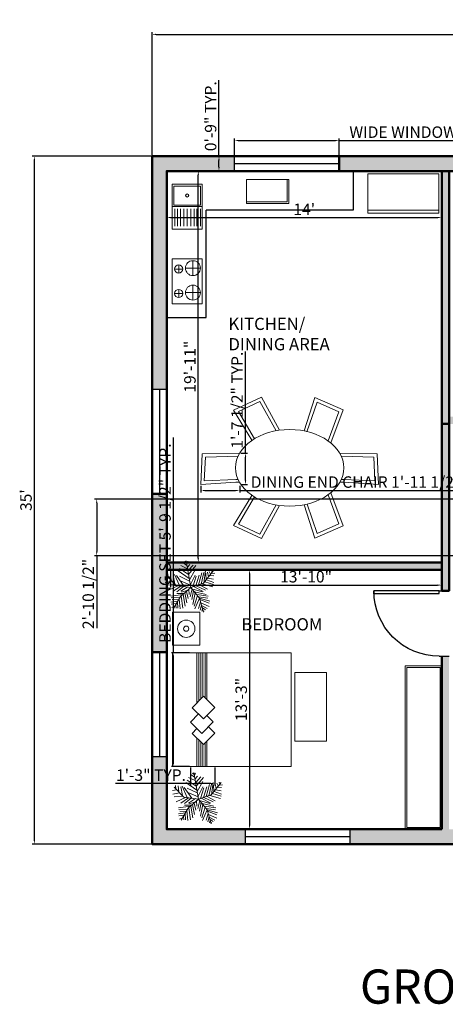
# Model space of a CAD drawing. Units: inches. Extents: x 1647 to 2354, y 1705 to 2321.
# Tile 1 of 4: x 1647 to 1907, y 1705 to 2307. Entities that reach past the tile are written whole.
import ezdxf

# ---------------------------------------------------------------- set-up
doc = ezdxf.new("R2010")
doc.units = ezdxf.units.IN
for name, color, linetype, lineweight in [('A-ANNO-DIMS', 130, 'Continuous', 18), ('A-ANNO-TEXT', 7, 'Continuous', 35), ('A-AREA-IDEN', 7, 'Continuous', 25), ('A-EQPM', 52, 'Continuous', 18), ('A-FLOR-CASE', 52, 'Continuous', 25), ('A-FLOR-FIXT', 52, 'Continuous', 18), ('A-WALL-PATT', 84, 'Continuous', 13), ('door', 142, 'Continuous', 25), ('fur', 52, 'Continuous', 18), ('tree', 92, 'Continuous', 13), ('wall', 84, 'Continuous', 50), ('window', 242, 'Continuous', 25)]:
    doc.layers.add(name, color=color, linetype=linetype, lineweight=lineweight)
doc.styles.get("Standard").update_dxf_attribs({"font": 'arial.ttf'})
doc.dimstyles.new('ISO-25', dxfattribs={"dimtxt": 7, "dimasz": 2.5, "dimexe": 1.25, "dimexo": 0.625, "dimtad": 1, "dimdec": 0, "dimlunit": 4, "dimtxsty": 'Standard', "dimcen": 2.5, "dimadec": 0, "dimazin": 0, "dimtfac": 1, "dimtdec": 0, "dimtmove": 0, "dimatfit": 3, "dimfxl": 1, "dimarcsym": 0})

# ---------------------------------------------------------------- blocks, each defined once
blk = doc.blocks.new('*U2')
for p, q in [((0, 0), (0, -6)), ((40, 0), (40, -6))]:
    blk.add_line(p, q)
blk.add_lwpolyline([(0, 0), (0, 40), (1.75, 40), (1.75, 0)], close=True)
blk.add_arc((0, 0), 40, 0, 90)
blk = doc.blocks.new('*U6')
for p, q in [((-7.288, 39.707), (-21.778, 46.673)), ((-8.737, 47.138), (-17.069, 52.711)), ((-10.186, 53.64), (-13.084, 55.962)), ((0, 0), (-10.5, 57)), ((-9.099, 51.782), (-6.563, 55.962)), ((-7.65, 43.423), (-2.578, 49.46)), ((-5.839, 35.992), (4.667, 48.067)), ((-5.114, 27.632), (10.463, 46.673)), ((-31.5, 4.5), (-52.5, 25.5)), ((-48.585, 21.131), (-49.309, 29.026)), ((-43.513, 28.561), (-42.427, 15.558)), ((-38.442, 26.239), (-34.819, 7.663)), ((-35.544, 28.097), (-24.314, 3.947)), ((-14.533, 2.09), (-30.834, 25.31)), ((-3.665, 19.273), (-27.574, 35.527)), ((-5.114, 28.097), (-24.676, 40.636)), ((-24.314, 23.917), (-2.941, 13.7)), ((-2.941, 16.486), (8.652, 37.85)), ((-1.129, 6.734), (9.014, 26.704)), ((3.942, 1.625), (11.187, 24.381)), ((10.101, 3.483), (17.708, 26.239)), ((16.259, 5.805), (23.142, 31.348)), ((22.055, 7.198), (27.489, 32.277)), ((27, 9), (48, 36)), ((27.127, 9.056), (31.112, 35.992)), ((31.836, 30.883), (32.561, 16.486)), ((35.096, 32.741), (37.27, 22.524)), ((38.719, 34.134), (41.979, 28.561)), ((40.53, 25.775), (48.862, 24.846)), ((43.791, 29.954), (51.036, 30.883)), ((44.153, 36.456), (45.239, 32.741)), ((-47.498, 19.737), (-55.83, 18.344)), ((-40.615, 13.7), (-55.105, 10.913)), ((-33.37, 6.269), (-52.207, 5.34)), ((-28.299, 3.483), (-47.86, -5.805)), ((-21.416, 3.018), (-38.079, -8.128)), ((0, 0), (-31.5, 4.5)), ((-15.982, 2.09), (-30.11, -9.521)), ((0, 0), (-22.5, -19.5)), ((-6.563, 1.161), (-21.416, -8.128)), ((-20.691, 13.7), (-1.129, 4.876)), ((0, 0), (27, 9)), ((0, 0), (18, -22.5)), ((6.478, 1.625), (26.04, -8.592)), ((11.187, 3.483), (30.749, -5.805)), ((18.07, 5.805), (35.096, -3.483)), ((24.229, 7.663), (46.688, 1.625)), ((29.662, 12.307), (48.137, 6.269)), ((33.285, 16.486), (48.862, 10.913)), ((36.183, 19.737), (48.137, 17.88)), ((-17.431, -15.094), (-42.789, -18.809)), ((-22.5, -19.5), (-37.5, -45)), ((-15.257, -12.772), (-30.11, -12.772)), ((-20.691, -18.345), (-17.793, -44.352)), ((-6.563, -5.805), (-19.967, -9.985)), ((-17.069, -15.094), (-12.721, -40.172)), ((-13.446, -11.378), (-8.737, -32.741)), ((-9.461, -8.592), (-6.201, -23.453)), ((-4.752, -3.483), (-3.665, -14.629)), ((2.493, -3.019), (-1.491, -20.202)), ((1.769, -2.555), (24.229, -9.521)), ((5.029, -6.27), (2.131, -25.775)), ((9.014, -11.378), (3.58, -35.992)), ((14.085, -16.951), (6.478, -40.172)), ((7.565, -9.056), (32.198, -14.629)), ((12.274, -15.094), (36.907, -18.809)), ((16.259, -19.738), (36.183, -22.989)), ((-28.299, -29.026), (-42.789, -31.348)), ((-24.314, -21.596), (-42.427, -22.06)), ((-30.834, -34.135), (-42.427, -35.528)), ((-34.457, -39.708), (-40.978, -42.494)), ((-26.849, -26.24), (-40.253, -25.775)), ((-32.646, -36.921), (-31.921, -44.352)), ((-29.023, -30.884), (-27.936, -43.887)), ((-25.038, -23.918), (-22.865, -45.281)), ((18.07, -22.524), (8.289, -45.745)), ((20.244, -30.419), (15.897, -44.816)), ((18, -22.5), (27, -52.5)), ((18.433, -22.524), (40.53, -29.026)), ((19.157, -25.311), (38.719, -33.206)), ((22.78, -37.85), (19.519, -48.532)), ((21.331, -32.741), (39.081, -40.636)), ((22.78, -38.314), (34.372, -44.816)), ((24.591, -45.745), (23.142, -50.854)), ((24.591, -43.423), (30.749, -47.603)), ((26.764, -49.925), (28.213, -50.854))]:
    blk.add_line(p, q)
blk = doc.blocks.new('*D7')
at = {"layer": 'A-ANNO-DIMS', "color": 0, "lineweight": -2, "transparency": 16777216}
for p, q in [((1737.13, 2213.61), (1737.13, 2184.55)), ((1905.13, 2213.61), (1905.13, 2184.55)), ((1739.63, 2185.8), (1902.63, 2185.8))]:
    blk.add_line(p, q, dxfattribs=at)
at = {"layer": 'A-ANNO-DIMS', "color": 0, "transparency": 16777216}
for points in [[(1739.63, 2186.21), (1739.63, 2185.38), (1737.13, 2185.8)], [(1902.63, 2186.21), (1902.63, 2185.38), (1905.13, 2185.8)]]:
    blk.add_solid(points, dxfattribs=at)
at = {"layer": 'Defpoints', "color": 0, "transparency": 16777216}
for p in [(1737.13, 2214.23), (1905.13, 2214.23), (1905.13, 2185.8)]:
    blk.add_point(p, dxfattribs=at)
at = {"layer": 'A-ANNO-DIMS', "color": 0, "transparency": 16777216, "insert": (1821.13, 2189.94), "char_height": 7, "attachment_point": 5}
blk.add_mtext("14'", dxfattribs=at)
blk = doc.blocks.new('*D8')
at = {"layer": 'A-ANNO-DIMS', "color": 0, "lineweight": -2, "transparency": 16777216}
for p, q in [((1737.76, 2214.23), (1757.65, 2214.23)), ((1756.4, 1977.73), (1756.4, 2211.73)), ((1737.76, 1975.23), (1757.65, 1975.23))]:
    blk.add_line(p, q, dxfattribs=at)
at = {"layer": 'A-ANNO-DIMS', "color": 0, "transparency": 16777216}
for points in [[(1755.98, 2211.73), (1756.81, 2211.73), (1756.4, 2214.23)], [(1755.98, 1977.73), (1756.81, 1977.73), (1756.4, 1975.23)]]:
    blk.add_solid(points, dxfattribs=at)
at = {"layer": 'Defpoints', "color": 0, "transparency": 16777216}
for p in [(1737.13, 2214.23), (1756.4, 2214.23), (1737.13, 1975.23)]:
    blk.add_point(p, dxfattribs=at)
at = {"layer": 'A-ANNO-DIMS', "color": 0, "transparency": 16777216, "insert": (1752.2, 2094.73), "char_height": 7, "attachment_point": 5, "rotation": 90}
blk.add_mtext('19\'-11"', dxfattribs=at)
blk = doc.blocks.new('*D13')
at = {"layer": 'A-ANNO-DIMS', "color": 0, "lineweight": -2, "transparency": 16777216}
for p, q in [((1739.39, 1970.11), (1739.39, 1960.1)), ((1905.13, 1970.11), (1905.13, 1960.1)), ((1741.89, 1961.35), (1902.63, 1961.35))]:
    blk.add_line(p, q, dxfattribs=at)
at = {"layer": 'A-ANNO-DIMS', "color": 0, "transparency": 16777216}
for points in [[(1741.89, 1961.76), (1741.89, 1960.93), (1739.39, 1961.35)], [(1902.63, 1961.76), (1902.63, 1960.93), (1905.13, 1961.35)]]:
    blk.add_solid(points, dxfattribs=at)
at = {"layer": 'Defpoints', "color": 0, "transparency": 16777216}
for p in [(1739.39, 1970.73), (1905.13, 1970.73), (1905.13, 1961.35)]:
    blk.add_point(p, dxfattribs=at)
at = {"layer": 'A-ANNO-DIMS', "color": 0, "transparency": 16777216, "insert": (1822.26, 1965.55), "char_height": 7, "attachment_point": 5}
blk.add_mtext('13\'-10"', dxfattribs=at)
blk = doc.blocks.new('*D14')
at = {"layer": 'A-ANNO-DIMS', "color": 0, "lineweight": -2, "transparency": 16777216}
for p, q in [((1737.76, 1970.73), (1788.98, 1970.73)), ((1787.73, 1968.23), (1787.73, 1814.73)), ((1737.76, 1812.23), (1788.98, 1812.23))]:
    blk.add_line(p, q, dxfattribs=at)
at = {"layer": 'A-ANNO-DIMS', "color": 0, "transparency": 16777216}
for points in [[(1787.32, 1968.23), (1788.15, 1968.23), (1787.73, 1970.73)], [(1787.32, 1814.73), (1788.15, 1814.73), (1787.73, 1812.23)]]:
    blk.add_solid(points, dxfattribs=at)
at = {"layer": 'Defpoints', "color": 0, "transparency": 16777216}
for p in [(1737.13, 1970.73), (1737.13, 1812.23), (1787.73, 1812.23)]:
    blk.add_point(p, dxfattribs=at)
at = {"layer": 'A-ANNO-DIMS', "color": 0, "transparency": 16777216, "insert": (1783.53, 1891.48), "char_height": 7, "attachment_point": 5, "rotation": 90}
blk.add_mtext('13\'-3"', dxfattribs=at)
blk = doc.blocks.new('*D24')
at = {"layer": 'A-ANNO-DIMS', "color": 0, "lineweight": -2, "transparency": 16777216}
for p, q in [((1728.13, 2223.86), (1728.13, 2298.93)), ((1730.63, 2297.68), (2265.63, 2297.68)), ((2268.13, 2223.86), (2268.13, 2298.93))]:
    blk.add_line(p, q, dxfattribs=at)
at = {"layer": 'A-ANNO-DIMS', "color": 0, "transparency": 16777216}
for points in [[(1730.63, 2298.09), (1730.63, 2297.26), (1728.13, 2297.68)], [(2265.63, 2298.09), (2265.63, 2297.26), (2268.13, 2297.68)]]:
    blk.add_solid(points, dxfattribs=at)
at = {"layer": 'Defpoints', "color": 0, "transparency": 16777216}
for p in [(2268.13, 2297.68), (1728.13, 2223.23), (2268.13, 2223.23)]:
    blk.add_point(p, dxfattribs=at)
at = {"layer": 'A-ANNO-DIMS', "color": 0, "transparency": 16777216, "insert": (1998.13, 2301.86), "char_height": 7, "attachment_point": 5}
blk.add_mtext("45'", dxfattribs=at)
blk = doc.blocks.new('*D25')
at = {"layer": 'A-ANNO-DIMS', "color": 0, "lineweight": -2, "transparency": 16777216}
for p, q in [((1727.51, 2223.23), (1654.99, 2223.23)), ((1656.24, 1805.73), (1656.24, 2220.73)), ((1727.51, 1803.23), (1654.99, 1803.23))]:
    blk.add_line(p, q, dxfattribs=at)
at = {"layer": 'A-ANNO-DIMS', "color": 0, "transparency": 16777216}
for points in [[(1655.82, 2220.73), (1656.66, 2220.73), (1656.24, 2223.23)], [(1655.82, 1805.73), (1656.66, 1805.73), (1656.24, 1803.23)]]:
    blk.add_solid(points, dxfattribs=at)
at = {"layer": 'Defpoints', "color": 0, "transparency": 16777216}
for p in [(1656.24, 2223.23), (1728.13, 2223.23), (1728.13, 1803.23)]:
    blk.add_point(p, dxfattribs=at)
at = {"layer": 'A-ANNO-DIMS', "color": 0, "transparency": 16777216, "insert": (1652.04, 2013.23), "char_height": 7, "attachment_point": 5, "rotation": 90}
blk.add_mtext("35'", dxfattribs=at)
blk = doc.blocks.new('WIN-WIDE-9IN-WALL')
blk.add_line((0, 4.5), (63.83, 4.5))
blk.add_lwpolyline([(0, 9), (63.83, 9), (63.83, 0), (0, 0)], close=True)
blk = doc.blocks.new('NIGHTSTAND-WITH-LAMP')
blk.add_lwpolyline([(0, 16.74), (20.08, 16.74), (20.08, 0), (0, 0)], close=True)
for radius in [5.31, 1.6]:
    blk.add_circle((10.04, 8.37), radius)
blk = doc.blocks.new('BED-PILLOW-AND-COVER-SET')
for p, q in [((0, 11.11), (17.43, 11.11)), ((0, 9.87), (16.21, 9.87)), ((0, 8.55), (14.92, 8.55)), ((0, 7.29), (13.67, 7.29)), ((38.64, 11.11), (69.38, 11.11)), ((39.89, 9.87), (69.38, 9.87)), ((41.22, 8.55), (69.38, 8.55)), ((42.51, 7.29), (69.38, 7.29)), ((0, 5.98), (14.28, 5.98)), ((0, 4.92), (15.36, 4.92)), ((31.01, 4.92), (31.05, 4.92)), ((40.88, 4.92), (69.38, 4.92)), ((41.93, 5.98), (69.38, 5.98))]:
    blk.add_line(p, q)
for points in [[(23.1, 10.95), (20.15, 13.86), (13.32, 6.93), (20.34, 0), (24.26, 3.97)], [(32.02, 9.99), (27.02, 14.92), (20.19, 7.99), (27.21, 1.06), (31.03, 4.93)]]:
    blk.add_lwpolyline(points)
blk.add_lwpolyline([(29.01, 6.93), (36.04, 0), (42.87, 6.93), (35.84, 13.86)], close=True)
blk = doc.blocks.new('BED-FOOT-BENCH')
blk.add_lwpolyline([(0, 19.36), (42.07, 19.36), (42.07, 0), (0, 0)], close=True)
blk = doc.blocks.new('DINING-CHAIR-END')
for p, q in [((0, 0), (0.72, 18.73)), ((0.72, 18.73), (23.74, 19.33)), ((2.75, 16.73), (2.11, 2.36)), ((22.72, 17.36), (2.75, 16.73)), ((21.45, 1.53), (0, 0)), ((21.29, 3.24), (2.11, 2.36)), ((21.29, 3.24), (22.7, 3.24)), ((21.45, 1.53), (23.57, 1.53))]:
    blk.add_line(p, q)
blk = doc.blocks.new('*D35')
at = {"layer": 'A-ANNO-DIMS', "color": 0, "lineweight": -2, "transparency": 16777216}
for p, q in [((1778.6, 2223.86), (1778.6, 2234.06)), ((1781.1, 2232.81), (1839.94, 2232.81)), ((1842.44, 2223.86), (1842.44, 2234.06)), ((1842.44, 2232.81), (1963.01, 2232.81))]:
    blk.add_line(p, q, dxfattribs=at)
at = {"layer": 'A-ANNO-DIMS', "color": 0, "transparency": 16777216}
for points in [[(1781.1, 2233.22), (1781.1, 2232.39), (1778.6, 2232.81)], [(1839.94, 2233.22), (1839.94, 2232.39), (1842.44, 2232.81)]]:
    blk.add_solid(points, dxfattribs=at)
at = {"layer": 'Defpoints', "color": 0, "transparency": 16777216}
for p in [(1842.44, 2232.81), (1778.6, 2223.23), (1842.44, 2223.23)]:
    blk.add_point(p, dxfattribs=at)
at = {"layer": 'A-ANNO-DIMS', "color": 0, "transparency": 16777216, "insert": (1903.97, 2237.05), "char_height": 7, "attachment_point": 5}
blk.add_mtext('WIDE WINDOW 5\'-4" TYP.', dxfattribs=at)
blk = doc.blocks.new('*D36')
at = {"layer": 'A-ANNO-DIMS', "color": 0, "lineweight": -2, "transparency": 16777216}
for p, q in [((1769.03, 2223.23), (1769.03, 2269.65)), ((1777.98, 2223.23), (1767.78, 2223.23)), ((1769.03, 2216.73), (1769.03, 2220.73)), ((1777.98, 2214.23), (1767.78, 2214.23))]:
    blk.add_line(p, q, dxfattribs=at)
at = {"layer": 'A-ANNO-DIMS', "color": 0, "transparency": 16777216}
for points in [[(1768.61, 2220.73), (1769.45, 2220.73), (1769.03, 2223.23)], [(1768.61, 2216.73), (1769.45, 2216.73), (1769.03, 2214.23)]]:
    blk.add_solid(points, dxfattribs=at)
at = {"layer": 'Defpoints', "color": 0, "transparency": 16777216}
for p in [(1769.03, 2223.23), (1778.6, 2223.23), (1778.6, 2214.23)]:
    blk.add_point(p, dxfattribs=at)
at = {"layer": 'A-ANNO-DIMS', "color": 0, "transparency": 16777216, "insert": (1764.83, 2247.69), "char_height": 7, "attachment_point": 5, "rotation": 90}
blk.add_mtext('0\'-9" TYP.', dxfattribs=at)
blk = doc.blocks.new('*D41')
at = {"layer": 'A-ANNO-DIMS', "color": 0, "lineweight": -2, "transparency": 16777216}
for p, q in [((1741.21, 1919.99), (1741.21, 2051.41)), ((1751, 1919.99), (1739.96, 1919.99)), ((1741.21, 1853.11), (1741.21, 1917.49)), ((1751, 1850.61), (1739.96, 1850.61))]:
    blk.add_line(p, q, dxfattribs=at)
at = {"layer": 'A-ANNO-DIMS', "color": 0, "transparency": 16777216}
for points in [[(1740.8, 1917.49), (1741.63, 1917.49), (1741.21, 1919.99)], [(1740.8, 1853.11), (1741.63, 1853.11), (1741.21, 1850.61)]]:
    blk.add_solid(points, dxfattribs=at)
at = {"layer": 'Defpoints', "color": 0, "transparency": 16777216}
for p in [(1741.21, 1919.99), (1751.62, 1919.99), (1751.62, 1850.61)]:
    blk.add_point(p, dxfattribs=at)
at = {"layer": 'A-ANNO-DIMS', "color": 0, "transparency": 16777216, "insert": (1736.97, 1986.95), "char_height": 7, "attachment_point": 5, "rotation": 90}
blk.add_mtext('BEDDING SET 5\'-9 1/2" TYP.', dxfattribs=at)
blk = doc.blocks.new('*D42')
at = {"layer": 'A-ANNO-DIMS', "color": 0, "lineweight": -2, "transparency": 16777216}
for p, q in [((1751.62, 1849.98), (1751.62, 1838.95)), ((1766.54, 1849.98), (1766.54, 1838.95)), ((1751.62, 1840.2), (1705.86, 1840.2)), ((1764.04, 1840.2), (1754.12, 1840.2))]:
    blk.add_line(p, q, dxfattribs=at)
at = {"layer": 'A-ANNO-DIMS', "color": 0, "transparency": 16777216}
for points in [[(1754.12, 1840.62), (1754.12, 1839.78), (1751.62, 1840.2)], [(1764.04, 1840.62), (1764.04, 1839.78), (1766.54, 1840.2)]]:
    blk.add_solid(points, dxfattribs=at)
at = {"layer": 'Defpoints', "color": 0, "transparency": 16777216}
for p in [(1751.62, 1850.61), (1766.54, 1850.61), (1751.62, 1840.2)]:
    blk.add_point(p, dxfattribs=at)
at = {"layer": 'A-ANNO-DIMS', "color": 0, "transparency": 16777216, "insert": (1727.49, 1844.4), "char_height": 7, "attachment_point": 5}
blk.add_mtext('1\'-3" TYP.', dxfattribs=at)
blk = doc.blocks.new('*D49')
at = {"layer": 'A-ANNO-DIMS', "color": 0, "lineweight": -2, "transparency": 16777216}
for p, q in [((1757.95, 2022.05), (1757.95, 2017.87)), ((1781.7, 2022.05), (1781.7, 2017.87)), ((1760.45, 2019.12), (1779.2, 2019.12)), ((1781.7, 2019.12), (1942.97, 2019.12))]:
    blk.add_line(p, q, dxfattribs=at)
at = {"layer": 'A-ANNO-DIMS', "color": 0, "transparency": 16777216}
for points in [[(1760.45, 2019.53), (1760.45, 2018.7), (1757.95, 2019.12)], [(1779.2, 2019.53), (1779.2, 2018.7), (1781.7, 2019.12)]]:
    blk.add_solid(points, dxfattribs=at)
at = {"layer": 'Defpoints', "color": 0, "transparency": 16777216}
for p in [(1757.95, 2022.68), (1781.7, 2022.68), (1781.7, 2019.12)]:
    blk.add_point(p, dxfattribs=at)
at = {"layer": 'A-ANNO-DIMS', "color": 0, "transparency": 16777216, "insert": (1863.58, 2023.36), "char_height": 7, "attachment_point": 5}
blk.add_mtext('DINING END CHAIR 1\'-11 1/2" TYP.', dxfattribs=at)
blk = doc.blocks.new('*D50')
at = {"layer": 'A-ANNO-DIMS', "color": 0, "lineweight": -2, "transparency": 16777216}
for p, q in [((1785.26, 2042.01), (1785.26, 2104.08)), ((1782.32, 2042.01), (1786.51, 2042.01)), ((1785.26, 2025.18), (1785.26, 2039.51)), ((1782.32, 2022.68), (1786.51, 2022.68))]:
    blk.add_line(p, q, dxfattribs=at)
at = {"layer": 'A-ANNO-DIMS', "color": 0, "transparency": 16777216}
for points in [[(1784.84, 2039.51), (1785.68, 2039.51), (1785.26, 2042.01)], [(1784.84, 2025.18), (1785.68, 2025.18), (1785.26, 2022.68)]]:
    blk.add_solid(points, dxfattribs=at)
at = {"layer": 'Defpoints', "color": 0, "transparency": 16777216}
for p in [(1781.7, 2042.01), (1785.26, 2042.01), (1781.7, 2022.68)]:
    blk.add_point(p, dxfattribs=at)
at = {"layer": 'A-ANNO-DIMS', "color": 0, "transparency": 16777216, "insert": (1781.01, 2074.29), "char_height": 7, "attachment_point": 5, "rotation": 90}
blk.add_mtext('1\'-7 1/2" TYP.', dxfattribs=at)
blk = doc.blocks.new('*D57')
at = {"layer": 'A-ANNO-DIMS', "color": 0, "lineweight": -2, "transparency": 16777216}
for p, q in [((2135.51, 2013.92), (1693.08, 2013.92)), ((1694.33, 2011.42), (1694.33, 1981.78)), ((2135.51, 1979.28), (1693.08, 1979.28)), ((1694.33, 1979.28), (1694.33, 1935.05))]:
    blk.add_line(p, q, dxfattribs=at)
at = {"layer": 'A-ANNO-DIMS', "color": 0, "transparency": 16777216}
for points in [[(1693.92, 2011.42), (1694.75, 2011.42), (1694.33, 2013.92)], [(1693.92, 1981.78), (1694.75, 1981.78), (1694.33, 1979.28)]]:
    blk.add_solid(points, dxfattribs=at)
at = {"layer": 'Defpoints', "color": 0, "transparency": 16777216}
for p in [(2136.13, 2013.92), (1694.33, 1979.28), (2136.13, 1979.28)]:
    blk.add_point(p, dxfattribs=at)
at = {"layer": 'A-ANNO-DIMS', "color": 0, "transparency": 16777216, "insert": (1690.09, 1955.92), "char_height": 7, "attachment_point": 5, "rotation": 90}
blk.add_mtext('2\'-10 1/2"', dxfattribs=at)

msp = doc.modelspace()

# ---------------------------------------------------------------- hatches: boundary and pattern name
at = {"layer": 'A-WALL-PATT'}
h = msp.add_hatch(color=256, dxfattribs=at)
h.dxf.hatch_style = 1
h.paths.add_polyline_path([(1737.13, 2214.23), (1778.6, 2214.23), (1778.6, 2223.23), (1728.13, 2223.23), (1728.13, 2080.92), (1737.13, 2080.92)])
h.paths.add_polyline_path([(1785.23, 1812.23), (1737.13, 1812.23), (1737.13, 1856.57), (1728.13, 1856.57), (1728.13, 1803.23), (1785.23, 1803.23)])
h.paths.add_polyline_path([(2020.88, 1812.23), (1967.48, 1812.23), (1967.48, 1803.23), (2020.88, 1803.23)])
h.paths.add_polyline_path([(2101.16, 1807.61), (2101.16, 1812.23), (2091.13, 1812.23), (2091.13, 1921.55), (2086.63, 1921.55), (2086.63, 1812.23), (2058.56, 1812.23), (2058.56, 1803.23), (2101.16, 1803.23)])
h.paths.add_polyline_path([(1929.8, 1812.23), (1909.63, 1812.23), (1909.63, 1848.23), (1909.63, 1917.89), (1905.13, 1917.89), (1905.13, 1812.23), (1882.72, 1812.23), (1849.06, 1812.23), (1849.06, 1803.23), (1929.8, 1803.23)])
h.paths.add_polyline_path([(2178.59, 1812.23), (2159.48, 1812.23), (2159.48, 1807.61), (2159.48, 1803.23), (2178.59, 1803.23)])
h.paths.add_polyline_path([(2268.13, 1856.83), (2259.13, 1856.83), (2259.13, 1815.23), (2259.13, 1812.23), (2242.42, 1812.23), (2242.42, 1803.23), (2268.13, 1803.23)])
h = msp.add_hatch(color=256, dxfattribs=at)
h.dxf.hatch_style = 1
h.paths.add_polyline_path([(1957.79, 2223.23), (1842.44, 2223.23), (1842.44, 2214.23), (1957.79, 2214.23)])
h.paths.add_polyline_path([(2147.66, 2223.23), (2021.62, 2223.23), (2021.62, 2214.23), (2147.66, 2214.23)])
h.paths.add_polyline_path([(2088.13, 2214.23), (2083.63, 2214.23), (2083.63, 2064.23), (2088.13, 2064.23)])
h.paths.add_polyline_path([(1909.63, 2214.23), (1905.13, 2214.23), (1905.13, 2059.73), (1909.63, 2059.73), (1909.63, 2064.23)])
h.paths.add_polyline_path([(1737.13, 2017.09), (1728.13, 2017.09), (1728.13, 1920.4), (1737.13, 1920.4)])
h.paths.add_polyline_path([(1905.13, 1975.23), (1737.13, 1975.23), (1737.13, 1970.73), (1905.13, 1970.73)])
h.paths.add_polyline_path([(1909.63, 2059.73), (1905.13, 2059.73), (1905.13, 1957.89), (1909.63, 1957.89)])
h.paths.add_polyline_path([(2036.41, 2064.23), (1909.63, 2064.23), (1909.63, 2059.73), (2036.41, 2059.73)])
h.paths.add_polyline_path([(2140.63, 1979.28), (2136.13, 1979.28), (2136.13, 1971.23), (2140.63, 1971.23)])
h.paths.add_polyline_path([(2136.13, 1975.73), (2091.13, 1975.73), (2091.13, 1971.23), (2136.13, 1971.23)])
h.paths.add_polyline_path([(2091.13, 1975.73), (2086.63, 1975.73), (2086.63, 1961.55), (2091.13, 1961.55)])
h.paths.add_polyline_path([(2259.13, 1975.73), (2140.63, 1975.73), (2140.63, 1971.23), (2259.13, 1971.23)])
h.paths.add_polyline_path([(2205.13, 2000.82), (2200.63, 2000.82), (2200.63, 1975.73), (2205.13, 1975.73)])
h.paths.add_polyline_path([(2268.13, 2111.84), (2259.13, 2111.84), (2259.13, 2036.03), (2268.13, 2036.03)])
h.paths.add_polyline_path([(2259.13, 2064.23), (2240.73, 2064.23), (2240.73, 2059.73), (2259.13, 2059.73)])
h.paths.add_polyline_path([(2268.13, 1998.35), (2259.13, 1998.35), (2259.13, 1989.23), (2259.13, 1920.66), (2268.13, 1920.66)])

# ---------------------------------------------------------------- linework, layer by layer
at = {"layer": 'A-EQPM'}
for p, q in [((1810.62, 2195.43), (1810.62, 2208.97)), ((1785.75, 2195.43), (1810.62, 2195.43)), ((1859.93, 2190.31), (1859.93, 2188.38)), ((1903.31, 2188.38), (1903.31, 2191.97)), ((1859.93, 2188.38), (1903.31, 2188.38)), ((1753.1, 2154.91), (1753.1, 2159.47)), ((1753.1, 2159.47), (1753.1, 2150.35)), ((1744.45, 2154.35), (1741.95, 2154.35)), ((1741.95, 2154.35), (1746.95, 2154.35)), ((1744.45, 2154.35), (1744.45, 2156.85)), ((1744.45, 2156.85), (1744.45, 2151.85)), ((1744.45, 2151.85), (1744.45, 2154.35)), ((1748.54, 2154.91), (1757.66, 2154.91)), ((1757.66, 2154.91), (1753.1, 2154.91)), ((1744.45, 2139.41), (1744.45, 2141.91)), ((1744.45, 2141.91), (1744.45, 2136.9)), ((1753.1, 2139.97), (1753.1, 2144.53)), ((1753.1, 2144.53), (1753.1, 2135.41)), ((1744.45, 2139.41), (1741.95, 2139.41)), ((1741.95, 2139.41), (1746.95, 2139.41)), ((1744.45, 2136.9), (1744.45, 2139.41)), ((1753.1, 2139.97), (1748.54, 2139.97)), ((1748.54, 2139.97), (1757.66, 2139.97)), ((1753.1, 2135.41), (1753.1, 2139.97))]:
    msp.add_line(p, q, dxfattribs=at)
for points in [[(1785.75, 2208.97), (1811.73, 2208.97), (1811.73, 2194.4), (1785.75, 2194.4)], [(1903.31, 2212.49), (1859.93, 2212.49), (1859.93, 2190.31), (1903.31, 2190.31)], [(1740.34, 2160.52), (1758.85, 2160.52), (1758.85, 2133.01), (1740.34, 2133.01)]]:
    msp.add_lwpolyline(points, close=True, dxfattribs=at)
for centre, radius in [((1753.1, 2154.91), 4.56), ((1744.45, 2154.35), 2.5), ((1744.45, 2139.41), 2.5), ((1753.1, 2139.97), 4.56)]:
    msp.add_circle(centre, radius, dxfattribs=at)
at = {"layer": 'A-FLOR-CASE'}
for p, q in [((1851.12, 2214.23), (1851.12, 2190.23)), ((1851.12, 2190.23), (1761.13, 2190.23)), ((1761.13, 2124.74), (1761.13, 2190.23)), ((1737.13, 2124.74), (1761.13, 2124.74))]:
    msp.add_line(p, q, dxfattribs=at)
at = {"layer": 'A-FLOR-FIXT'}
for p, q in [((1740.34, 2192.49), (1758.85, 2192.49)), ((1742.08, 2180.57), (1742.08, 2191.03)), ((1743.72, 2180.57), (1743.72, 2191.03)), ((1745.6, 2180.57), (1745.6, 2191.03)), ((1747.53, 2180.57), (1747.53, 2191.03)), ((1749.64, 2180.57), (1749.64, 2191.03)), ((1751.75, 2180.57), (1751.75, 2191.03)), ((1753.82, 2180.57), (1753.82, 2191.03)), ((1755.6, 2180.57), (1755.6, 2191.03)), ((1757.67, 2180.57), (1757.67, 2191.03))]:
    msp.add_line(p, q, dxfattribs=at)
for points in [[(1740.34, 2206.24), (1758.85, 2206.24), (1758.85, 2178.73), (1740.34, 2178.73)], [(1741.53, 2193.41), (1757.73, 2193.41), (1757.73, 2205.07), (1741.53, 2205.07)]]:
    msp.add_lwpolyline(points, close=True, dxfattribs=at)
msp.add_circle((1749.63, 2199.24), 0.949, dxfattribs=at)
at = {"layer": 'fur'}
for p, q in [((1777.96, 2068.1), (1794.92, 2076.1)), ((1794.92, 2076.1), (1806.06, 2055.94)), ((1821.16, 2055.48), (1827.68, 2075.97)), ((1827.68, 2075.97), (1844.82, 2068.36)), ((1794.07, 2073.37), (1781.02, 2067.31)), ((1804.02, 2055.62), (1794.07, 2073.37)), ((1822.8, 2054.99), (1829.09, 2073.14)), ((1842.2, 2067.22), (1829.09, 2073.14)), ((1789.2, 2049.77), (1777.96, 2068.1)), ((1790.64, 2050.7), (1781.02, 2067.31)), ((1835.74, 2049.4), (1842.2, 2067.22)), ((1844.82, 2068.36), (1837.36, 2048.16)), ((1790.64, 2050.7), (1789.5, 2049.97)), ((1789.2, 2016.14), (1777.96, 1997.81)), ((1790.64, 2015.21), (1781.02, 1998.59)), ((1835.74, 2016.51), (1842.2, 1998.69)), ((1844.82, 1997.55), (1837.36, 2017.75)), ((1804.02, 2010.29), (1794.07, 1992.54)), ((1794.92, 1989.81), (1806.06, 2009.97)), ((1821.16, 2010.43), (1827.68, 1989.94)), ((1822.84, 2010.8), (1829.09, 1992.77)), ((1777.96, 1997.81), (1794.92, 1989.81)), ((1794.07, 1992.54), (1781.02, 1998.59)), ((1827.68, 1989.94), (1844.82, 1997.55)), ((1842.2, 1998.69), (1829.09, 1992.77))]:
    msp.add_line(p, q, dxfattribs=at)
for points in [[(1740.66, 1850.61), (1740.66, 1919.99), (1813.17, 1919.99), (1813.17, 1850.61)], [(1905.13, 1912.06), (1882.72, 1912.06), (1882.72, 1812.23), (1905.13, 1812.23)], [(1904.13, 1911.06), (1883.72, 1911.06), (1883.72, 1813.23), (1904.13, 1813.23)]]:
    msp.add_lwpolyline(points, close=True, dxfattribs=at)
msp.add_ellipse((1812.21, 2032.95), major_axis=(33.09, 0), ratio=0.706873, dxfattribs=at)
at = {"layer": 'wall'}
for p, q in [((1728.13, 2223.23), (2268.13, 2223.23)), ((1728.13, 1803.23), (1728.13, 2223.23)), ((1737.13, 2214.23), (1905.13, 2214.23)), ((1905.13, 2214.23), (1905.13, 1975.23)), ((1905.13, 1975.23), (1737.13, 1975.23)), ((1905.13, 1970.73), (1737.13, 1970.73)), ((1905.13, 1970.73), (1905.13, 1957.89)), ((1905.13, 1917.89), (1905.13, 1812.23)), ((2101.16, 1803.23), (1728.13, 1803.23))]:
    msp.add_line(p, q, dxfattribs=at)
for points in [[(2101.16, 1803.23), (1728.13, 1803.23), (1728.13, 2223.23), (2268.13, 2223.23), (2268.13, 1803.23), (2159.48, 1803.23)], [(1737.13, 1975.23), (1737.13, 2214.23), (1905.13, 2214.23)], [(1905.13, 1812.23), (1737.13, 1812.23), (1737.13, 1970.73)]]:
    msp.add_lwpolyline(points, dxfattribs=at)
for points in [[(1842.44, 2223.23), (1957.79, 2223.23), (1957.79, 2214.23), (1842.44, 2214.23)], [(1905.13, 2214.23), (1909.63, 2214.23), (1909.63, 2059.73), (1905.13, 2059.73)], [(1905.13, 1957.89), (1909.63, 1957.89), (1909.63, 2059.73), (1905.13, 2059.73)], [(1728.13, 1920.4), (1737.13, 1920.4), (1737.13, 2017.09), (1728.13, 2017.09)], [(1737.13, 1970.73), (1905.13, 1970.73), (1905.13, 1975.23), (1737.13, 1975.23)]]:
    msp.add_lwpolyline(points, close=True, dxfattribs=at)

# ---------------------------------------------------------------- block references
at = {"layer": 'door', "xscale": -1, "rotation": 90}
msp.add_blockref('*U2', (1903.63, 1957.89), dxfattribs=at)
at = {"layer": 'fur'}
msp.add_blockref('DINING-CHAIR-END', (1757.95, 2022.68), dxfattribs=at)
at = {"layer": 'fur', "extrusion": (0, 0, -1), "zscale": -1}
msp.add_blockref('DINING-CHAIR-END', (-1866.47, 2022.68), dxfattribs=at)
at = {"layer": 'fur'}
for name, p, rotation in [('NIGHTSTAND-WITH-LAMP', (1757.4, 1924.68), 89.99999999999989), ('BED-PILLOW-AND-COVER-SET', (1766.54, 1850.61), 89.99999999999945), ('BED-FOOT-BENCH', (1834.78, 1865.96), 90.00000000000006)]:
    msp.add_blockref(name, p, dxfattribs=dict(at, rotation=rotation))
at = {"layer": 'tree', "xscale": 0.2858091163346259, "yscale": 0.2858091163346259, "zscale": 0.2858091163346259}
for p in [(1751.94, 1959.88), (1756.62, 1830.6)]:
    msp.add_blockref('*U6', p, dxfattribs=at)
at = {"layer": 'window'}
for p in [(1778.61, 2214.23), (1785.23, 1803.23)]:
    msp.add_blockref('WIN-WIDE-9IN-WALL', p, dxfattribs=at)
for p, rotation in [((1728.13, 2080.92), 270.0000000000007), ((1728.13, 1920.4), 270.0000000000006)]:
    msp.add_blockref('WIN-WIDE-9IN-WALL', p, dxfattribs=dict(at, rotation=rotation))

# ---------------------------------------------------------------- texts
at = {"layer": 'A-ANNO-TEXT', "insert": (1855.17, 1726.6), "char_height": 20.8881, "attachment_point": 1}
msp.add_mtext_dynamic_manual_height_columns('GROUND FLOOR PLAN', width=3558.7841, gutter_width=104.44, heights=[0], dxfattribs=at)
at = {"layer": 'A-AREA-IDEN', "attachment_point": 1}
for s, insert, char_height in [('KITCHEN/\\PDINING AREA', (1774.84, 2124.62), 7.4646), ('BEDROOM', (1782.69, 1941.13), 7.465)]:
    msp.add_mtext_dynamic_manual_height_columns(s, width=263.8302, gutter_width=37.32, heights=[0], dxfattribs=dict(at, insert=insert, char_height=char_height))

# ---------------------------------------------------------------- dimensions: what is measured, and where the dimension line sits
at = {"layer": 'A-ANNO-DIMS'}
for base, p1, p2, picture, middle in [((2268.13, 2297.68), (1728.13, 2223.23), (2268.13, 2223.23), '*D24', (1998.13, 2301.86)), ((1905.13, 2185.8), (1737.13, 2214.23), (1905.13, 2214.23), '*D7', (1821.13, 2189.94)), ((1905.13, 1961.35), (1739.39, 1970.73), (1905.13, 1970.73), '*D13', (1822.26, 1965.55))]:
    dim = msp.add_linear_dim(base=base, p1=p1, p2=p2, dimstyle='ISO-25', override={"dimclrd": 0, "dimclre": 0, "dimclrt": 0}, dxfattribs=at)
    dim.commit()
    dim.dimension.update_dxf_attribs({"geometry": picture, "text_midpoint": middle})
for base, p1, p2, angle, text, picture, middle in [((1769.03, 2223.23), (1778.6, 2214.23), (1778.6, 2223.23), 90, '<> TYP.', '*D36', (1764.83, 2247.69)), ((1785.26, 2042.01), (1781.7, 2022.68), (1781.7, 2042.01), 90, '<> TYP.', '*D50', (1781.01, 2074.29)), ((1741.21, 1919.99), (1751.62, 1850.61), (1751.62, 1919.99), 90, 'BEDDING SET <> TYP.', '*D41', (1736.97, 1986.95)), ((1751.62, 1840.2), (1766.54, 1850.61), (1751.62, 1850.61), 180, '<> TYP.', '*D42', (1727.49, 1844.4))]:
    dim = msp.add_linear_dim(base=base, p1=p1, p2=p2, angle=angle, text=text, dimstyle='ISO-25', override={"dimdec": 1, "dimlfac": 1, "dimrnd": 0, "dimzin": 1, "dimdsep": 46, "dimlunit": 4, "dimfrac": 2}, dxfattribs=at)
    dim.commit()
    dim.dimension.update_dxf_attribs({"geometry": picture, "text_midpoint": middle})
for base, p1, p2, text, picture, middle in [((1842.44, 2232.81), (1778.6, 2223.23), (1842.44, 2223.23), 'WIDE WINDOW <> TYP.', '*D35', (1903.97, 2237.05)), ((1781.6967, 2019.1164), (1757.952, 2022.6781), (1781.6967, 2022.6781), 'DINING END CHAIR <> TYP.', '*D49', (1863.5812, 2023.3608))]:
    dim = msp.add_linear_dim(base=base, p1=p1, p2=p2, text=text, dimstyle='ISO-25', override={"dimdec": 1, "dimlfac": 1, "dimrnd": 0, "dimzin": 1, "dimdsep": 46, "dimlunit": 4, "dimfrac": 2}, dxfattribs=at)
    dim.commit()
    dim.dimension.update_dxf_attribs({"geometry": picture, "text_midpoint": middle})
for base, p1, p2, override, picture, middle in [((1656.24, 2223.23), (1728.13, 1803.23), (1728.13, 2223.23), {"dimclrd": 0, "dimclre": 0, "dimclrt": 0}, '*D25', (1652.04, 2013.23)), ((1756.4, 2214.23), (1737.13, 1975.23), (1737.13, 2214.23), {"dimclrd": 0, "dimclre": 0, "dimclrt": 0}, '*D8', (1752.2, 2094.73)), ((1694.33, 1979.28), (2136.13, 2013.92), (2136.13, 1979.28), {"dimdec": 1, "dimlfac": 1, "dimrnd": 0, "dimzin": 1, "dimdsep": 46, "dimlunit": 4, "dimfrac": 2}, '*D57', (1690.09, 1955.92)), ((1787.73223002, 1812.23275818), (1737.13438186, 1970.73275818), (1737.13438186, 1812.23275818), {"dimclrd": 0, "dimclre": 0, "dimclrt": 0}, '*D14', (1783.53083165, 1891.48275818))]:
    dim = msp.add_linear_dim(base=base, p1=p1, p2=p2, angle=90, dimstyle='ISO-25', override=override, dxfattribs=at)
    dim.commit()
    dim.dimension.update_dxf_attribs({"geometry": picture, "text_midpoint": middle})

doc.saveas('drawing.dxf')
